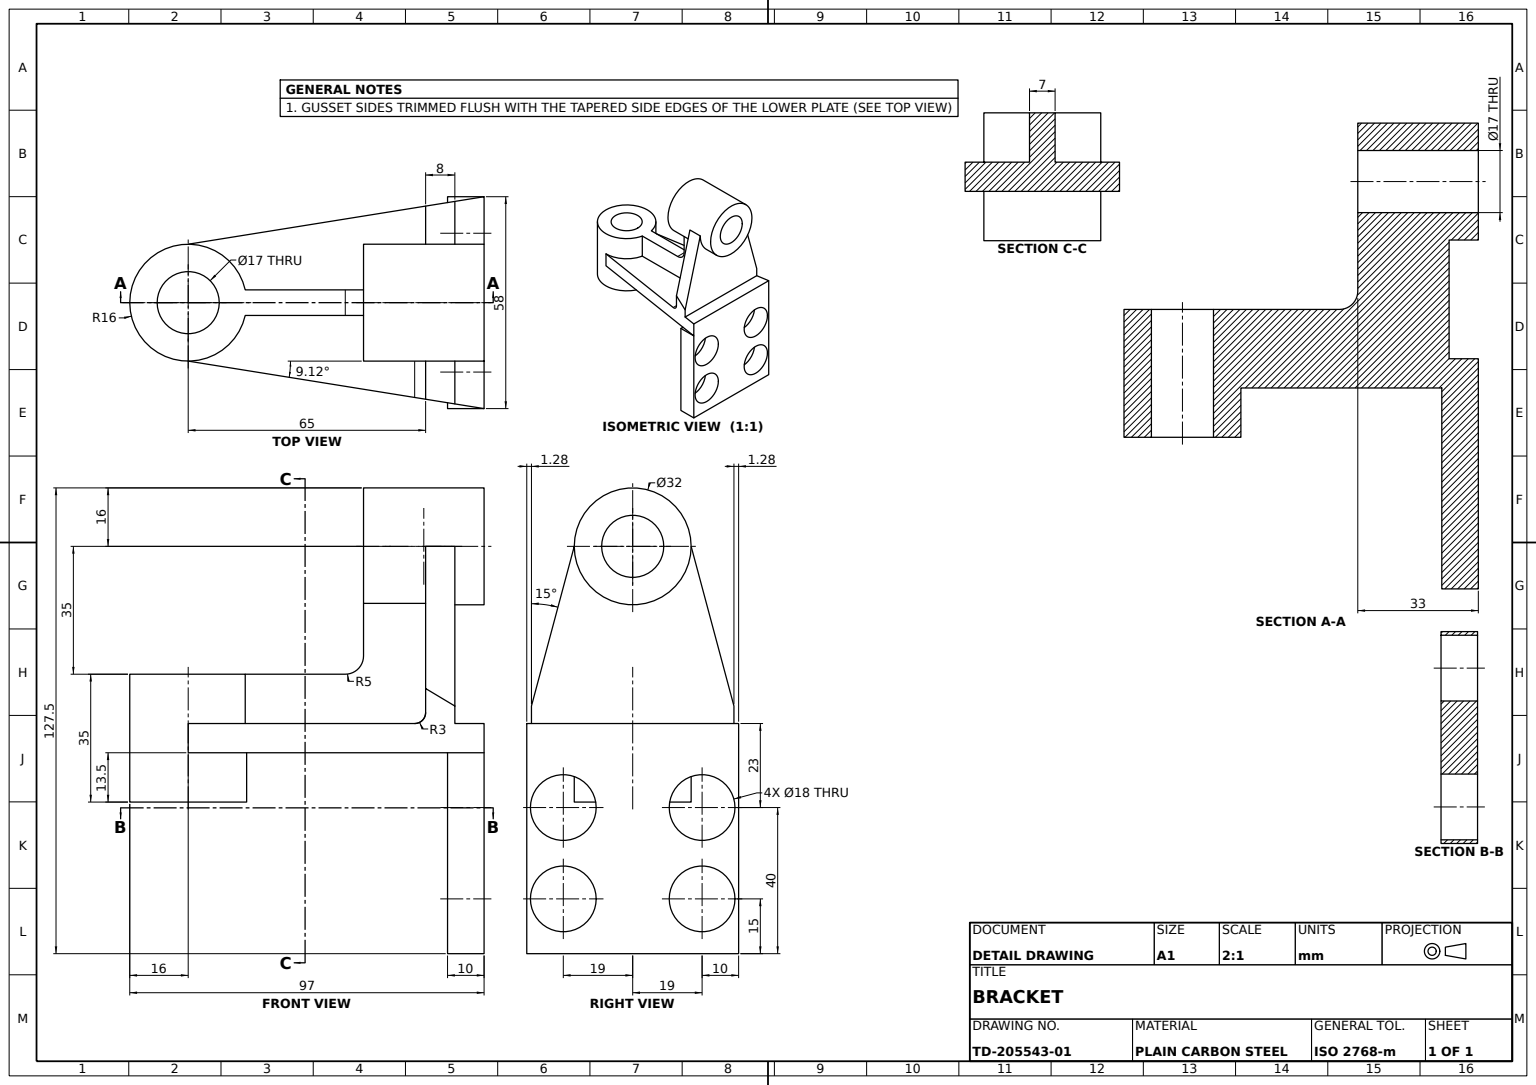
SolidWorks part; units mm, degrees
material "Plain Carbon Steel"
ref_plane "Front Plane" through (0, 0, 0) normal (0, 0, 1) x (1, 0, 0)
ref_plane "Top Plane" through (0, 0, 0) normal (0, 1, 0) x (1, 0, 0)
ref_plane "Right Plane" through (0, 0, 0) normal (1, 0, 0) x (0, 0, -1)
sketch "Main Boss Sketch Ø32" plane through (0, 0, 0) normal (0, 1, 0) x (1, 0, 0)
  circle A0 centre (0, 0) radius 16
  dimension "D1" = 32
extrude "Main Boss Ø32" add sketch "Main Boss Sketch Ø32" against normal mid plane 35
sketch "Main Boss Bore Sketch" plane through (0, 17.5, 0) normal (0, 1, 0) x (1, 0, 0)
  circle A0 centre (0, 0) radius 8.5
  dimension "D1" = 17
extrude "Main Boss Bore" cut sketch "Main Boss Bore Sketch" against normal blind 57
sketch "Lower Arm Sketch" plane through (0, 0, 0) normal (0, 1, 0) x (1, 0, 0)
  line L1 (0, 81) -> (29, 81)
  line L2 (29, 81) -> (16, 0)
  line L3 (0, 81) -> (-29, 81)
  line L4 (-29, 81) -> (-16, 0)
  circle A0 centre (0, 0) radius 16 construction
  arc A1 (16, 0) -> (-16, 0) centre (0, 0) ccw
  dimension "D1" = 29
  dimension "D2" = 81
extrude "Lower Arm Plate" add sketch "Lower Arm Sketch" along normal mid plane 8
ref_plane "Plane1" through (0, 0, -48) normal (0, 0, 1) x (1, 0, 0)
sketch "Upper Boss Sketch" plane through (0, 0, -48) normal (0, 0, 1) x (1, 0, 0)
  line L0 (0, 17.5) -> (0, 52.5)
  line L1 (8.5, 17.5) -> (-8.5, 17.5) construction
  circle A0 centre (0, 52.5) radius 16
  dimension "D1" = 32
  dimension "D2" = 35
extrude "Upper Boss" add sketch "Upper Boss Sketch" against normal blind 33 separate body
sketch "Upper Boss Bore Sketch" plane through (0, 0, -48) normal (0, 0, 1) x (1, 0, 0)
  circle A0 centre (0, 52.5) radius 8.5
  dimension "D1" = 17
extrude "Upper Boss Bore" cut sketch "Upper Boss Bore Sketch" against normal blind 38
ref_plane "Plane2" through (0, 0, -65) normal (0, 0, 1) x (1, 0, 0)
sketch "Upper Arm Sketch" plane through (0, 0, -65) normal (0, 0, 1) x (1, 0, 0)
  line L1 (-26.4317, 4) -> (29, 4)
  line L3 (-16, 52.5) -> (-29, 4)
  line L4 (-29, 4) -> (-26.4317, 4)
  line L5 (16, 52.5) -> (29, 4)
  circle A0 centre (0, 52.5) radius 16 construction
  arc A1 (-16, 52.5) -> (16, 52.5) centre (0, 52.5) ccw
  dimension "D1" = 2.5683
extrude "Upper Arm Plate" add sketch "Upper Arm Sketch" against normal blind 8
sketch "Plate Cut Set A Sketch" plane through (0, -4, 0) normal (0, -1, 0) x (1, 0, 0)
  line L0 (27.716, -73) -> (26.4321, -65)
  line L1 (31.9, -65) -> (-31.9, -65) construction
  line L2 (26.4321, -65) -> (27.716, -73) construction
  line L3 (26.4321, -65) -> (29, -65)
  line L4 (29, -73) -> (29, -65) construction
  line L5 (29, -65) -> (29, -73)
  line L6 (29, -73) -> (27.716, -73)
extrude "Plate Cut Set A" cut sketch "Plate Cut Set A Sketch" against normal blind 38
sketch "Plate Cut Set B Sketch" plane through (0, -4, 0) normal (0, -1, 0) x (1, 0, 0)
  line L0 (-26.4321, -65) -> (-29, -65)
  line L1 (-29, -65) -> (-29, -73)
  line L2 (-29, -73) -> (-27.716, -73)
  line L3 (-29, -81) -> (-16, 0) construction
  line L4 (-29, -73) -> (-27.716, -73) construction
  line L5 (-27.716, -73) -> (-26.4321, -65)
extrude "Plate Cut Set B" cut sketch "Plate Cut Set B Sketch" against normal blind 38
sketch "Rib Sketch" plane through (0, 0, 0) normal (1, 0, 0) x (0, 0, -1)
  line L0 (48, 17.5) -> (11.2691, 17.5)
  line L1 (48, 40.0023) -> (48, 17.5)
  line L2 (48, 68.5) -> (48, 36.5) construction
  line L3 (16, 17.5) -> (-16, 17.5) construction
  line L4 (11.2691, 17.5) -> (11.2691, 4)
  line L5 (0, 4) -> (65, 4) construction
  line L6 (11.2691, 4) -> (65, 4)
  line L7 (65, 4) -> (65, 40.0023)
  line L8 (65, 52.5) -> (65, 36.5) construction
  line L9 (65, 40.0023) -> (48, 40.0023)
  dimension "D1" = 36.7309
  dimension "D2" = 36.0023
extrude "Rib" add sketch "Rib Sketch" along normal mid plane 7
fillet "Rib Fillet R5" radius 5 1 edges at (0, 17.5, -48)
fillet "Arm Junction Fillet R3" radius 3 1 edges at (14.966, 4, -65)
sketch "Gusset Sketch" plane through (0, -4, 0) normal (0, -1, 0) x (1, 0, 0)
  line L0 (0, -81) -> (29, -81)
  line L1 (29, -81) -> (-29, -81) construction
  line L2 (29, -81) -> (29, -71)
  line L3 (29, -71) -> (-29, -71)
  line L4 (-29, -71) -> (-29, -81)
  line L5 (-29, -81) -> (29, -81)
  dimension "D1" = 10
extrude "Gusset" add sketch "Gusset Sketch" along normal blind 55 contours L2 L3 L4 L5
sketch "Gusset Trim Sketch" plane through (0, 0, -71) normal (0, 0, 1) x (1, 0, 0)
  line L0 (27.3951, -4) -> (-27.3951, -4) construction
  circle A0 centre (19, -44) radius 9
  circle A1 centre (19, -19) radius 9
  circle A2 centre (-19, -44) radius 9
  circle A3 centre (-19, -19) radius 9
  dimension "D1" = 18
  dimension "D2" = 10
  dimension "D3" = 48
  dimension "D4" = 15
  dimension "D5" = 40
extrude "Gusset Trim Cut" cut sketch "Gusset Trim Sketch" against normal blind 55
